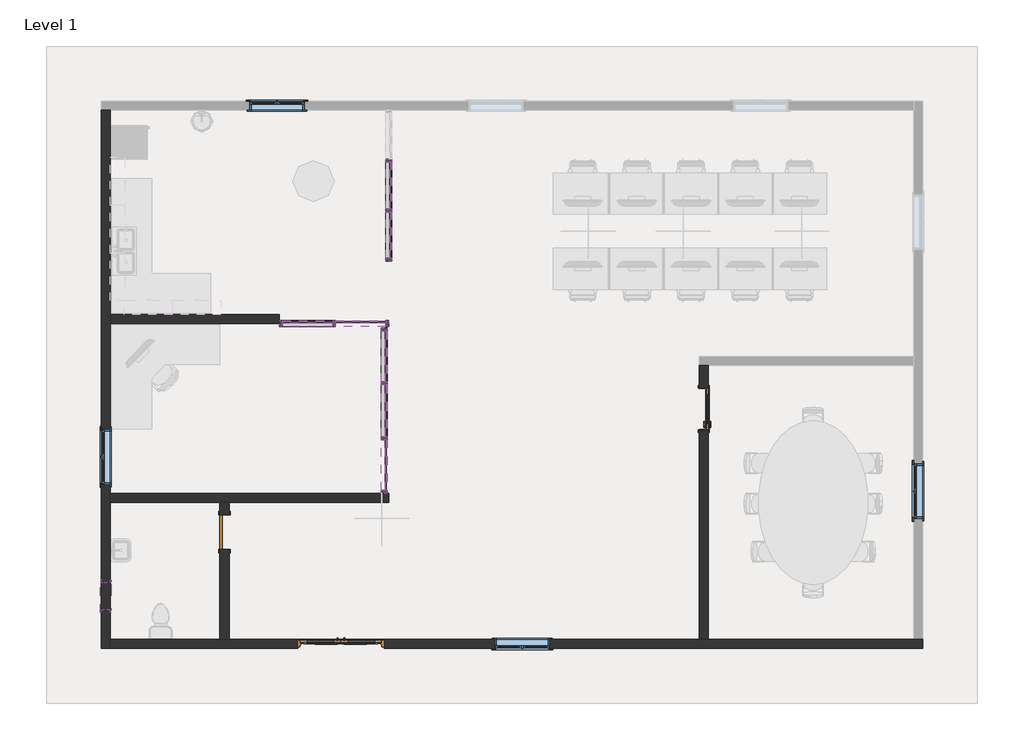
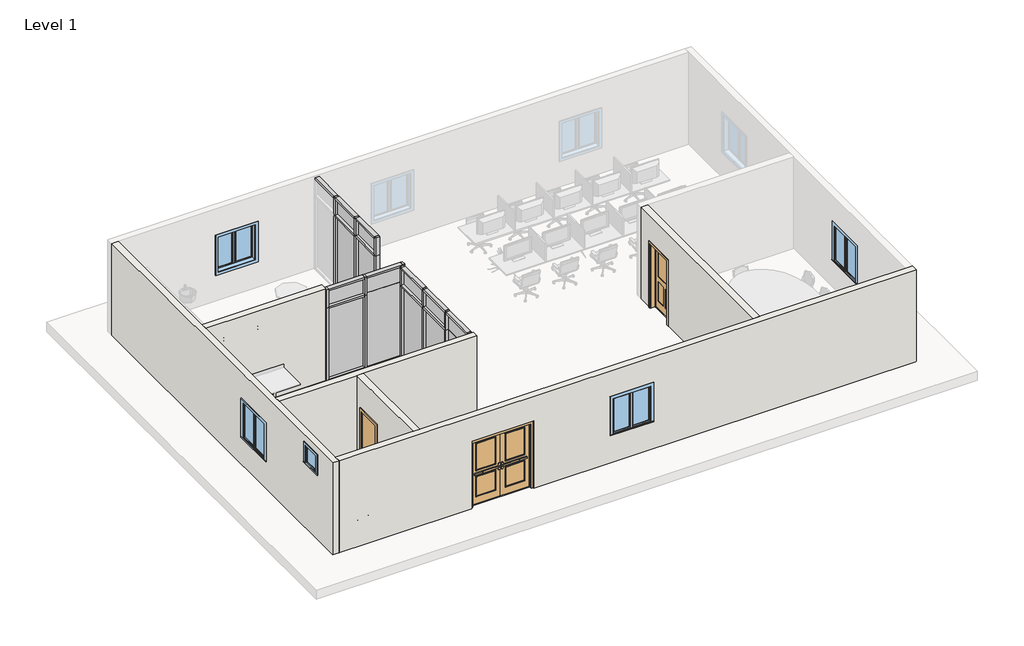
# One storey, part 1 of 2: 38 members, 14 plates, 6 walls, 5 windows, 3 doors.
"""IFC4 building model written with IfcOpenShell, lengths in millimetres."""

from ifc_helpers import new_model, si_unit, frame, origin, origin_with_axes, place, context, project, spatial, polyline, outline, extrude, faceted_brep, transform, mapped, element, save
from components import door_3d09584f, door_6260e01d, door_549a8064, door_95a5efb1, door_1a782ffc, member_f0fea5a5, member_6e77e263, member_47bfaf8a, member_ee409385, member_43f490c4, member_f0038585, member_e3a8255e, member_ffab42ea, member_e6b9f524, member_866a01fa, member_a1c24a98, member_7fa39cca, member_38455fd9, member_afdd3af2, system_panel_glazed_bba99bb7, system_panel_glazed_3d427df9, system_panel_glazed_c20df1b6, system_panel_glazed_49ccfb91, system_panel_glazed_2148303e, system_panel_glazed_80d043f3, system_panel_glazed_79634188, system_panel_glazed_0c115810, system_panel_glazed_47378ea7, system_panel_glazed_21725642, system_panel_glazed_958d1135, system_panel_glazed_0266aec6, system_panel_glazed_6663e6a9, system_panel_glazed_40ca61d7, window_0862ab64, window_e41d21a6

model = new_model("IFC4")

# Units and contexts
model_context = context("Model", 3, world=origin())
ifc_project = project(units=[si_unit("LENGTHUNIT", "METRE", prefix="MILLI")], contexts=[model_context])

# Site, building, storey
site = spatial("IfcSite", under=ifc_project)
building = spatial("IfcBuilding", under=site)
storey = spatial("IfcBuildingStorey", under=building, Name="Level 1", Elevation=0.0)

# Doors
placement = place(None, origin())
door_shape = door_3d09584f(model_context)
element("IfcDoor", 1, ObjectType="36\" x 84\"", at=placement, inside=storey, context=model_context, shape_type="MappedRepresentation", body=[
    mapped(door_shape, transform((-3033.298902, -683.2685778, 0.0), x_axis=(0.0, -1.0, 0.0), y_axis=(1.0, 0.0, 0.0), z_axis=(0.0, 0.0, 1.0))),
])
door_2_shape = door_6260e01d(model_context)
door_3_shape = door_549a8064(model_context)
door_4_shape = door_95a5efb1(model_context)
element("IfcDoor", 2, ObjectType="Door-Exterior-Double-Two_Lite : 72\" x 84\"", at=placement, inside=storey, context=model_context, shape_type="MappedRepresentation", body=[
    mapped(door_2_shape, transform((-11113.673902, -5922.0185778, 0.0), x_axis=(1.0, 0.0, 0.0), y_axis=(0.0, 1.0, 0.0), z_axis=(0.0, 0.0, 1.0))),
    mapped(door_3_shape, transform((-11113.673902, -5922.0185778, 0.0), x_axis=(1.0, 0.0, 0.0), y_axis=(0.0, 1.0, 0.0), z_axis=(0.0, 0.0, 1.0))),
    mapped(door_4_shape, transform((-11113.673902, -5922.0185778, 0.0), x_axis=(1.0, 0.0, 0.0), y_axis=(0.0, 1.0, 0.0), z_axis=(0.0, 0.0, 1.0))),
])
door_5_shape = door_1a782ffc(model_context)
element("IfcDoor", 3, ObjectType="Door-Single-Panel : 30\" x 80\"", at=placement, inside=storey, context=model_context, shape_type="MappedRepresentation", body=[
    mapped(door_5_shape, transform((-13704.473902, -3426.4685778, 0.0), x_axis=(0.0, 1.0, 0.0), y_axis=(-1.0, 0.0, 0.0), z_axis=(0.0, 0.0, 1.0))),
])

# Members
member_shape = member_f0fea5a5(model_context)
element("IfcMember", 4, ObjectType="Rectangular Mullion : 2.5\" x 5\" rectangular", at=placement, inside=storey, context=model_context, shape_type="MappedRepresentation", body=[
    mapped(member_shape, transform((-10148.473902, -107.5352444, 0.0), x_axis=(0.0, -1.0, 0.0), y_axis=(-1.0, 0.0, 0.0), z_axis=(0.0, 0.0, -1.0))),
])
element("IfcMember", 5, ObjectType="Rectangular Mullion : 2.5\" x 5\" rectangular", at=placement, inside=storey, context=model_context, shape_type="MappedRepresentation", body=[
    mapped(member_shape, transform((-10148.473902, -1335.2019111, 0.0), x_axis=(0.0, -1.0, 0.0), y_axis=(-1.0, 0.0, 0.0), z_axis=(0.0, 0.0, -1.0))),
])
element("IfcMember", 6, ObjectType="Rectangular Mullion : 2.5\" x 5\" rectangular", at=placement, inside=storey, context=model_context, shape_type="MappedRepresentation", body=[
    mapped(member_shape, transform((-11266.073902, 1221.7314222, 0.0), x_axis=(1.0, 0.0, 0.0), y_axis=(0.0, -1.0, 0.0), z_axis=(0.0, 0.0, -1.0))),
])
element("IfcMember", 7, ObjectType="Rectangular Mullion : 2.5\" x 5\" rectangular", at=placement, inside=storey, context=model_context, shape_type="MappedRepresentation", body=[
    mapped(member_shape, transform((-10046.873902, 4853.9314222, 0.0), x_axis=(0.0, -1.0, 0.0), y_axis=(-1.0, 0.0, 0.0), z_axis=(0.0, 0.0, -1.0))),
])
element("IfcMember", 8, ObjectType="Rectangular Mullion : 2.5\" x 5\" rectangular", at=placement, inside=storey, context=model_context, shape_type="MappedRepresentation", body=[
    mapped(member_shape, transform((-10046.873902, 3736.3314222, 0.0), x_axis=(0.0, -1.0, 0.0), y_axis=(-1.0, 0.0, 0.0), z_axis=(0.0, 0.0, -1.0))),
])
member_2_shape = member_6e77e263(model_context)
element("IfcMember", 9, ObjectType="Rectangular Mullion : 2.5\" x 5\" rectangular", at=placement, inside=storey, context=model_context, shape_type="MappedRepresentation", body=[
    mapped(member_2_shape, transform((-10148.473902, -107.5352444, 2438.4), x_axis=(0.0, -1.0, 0.0), y_axis=(-1.0, 0.0, 0.0), z_axis=(0.0, 0.0, -1.0))),
])
element("IfcMember", 10, ObjectType="Rectangular Mullion : 2.5\" x 5\" rectangular", at=placement, inside=storey, context=model_context, shape_type="MappedRepresentation", body=[
    mapped(member_2_shape, transform((-10148.473902, -1335.2019111, 2438.4), x_axis=(0.0, -1.0, 0.0), y_axis=(-1.0, 0.0, 0.0), z_axis=(0.0, 0.0, -1.0))),
])
element("IfcMember", 11, ObjectType="Rectangular Mullion : 2.5\" x 5\" rectangular", at=placement, inside=storey, context=model_context, shape_type="MappedRepresentation", body=[
    mapped(member_2_shape, transform((-11266.073902, 1221.7314222, 2438.4), x_axis=(1.0, 0.0, 0.0), y_axis=(0.0, -1.0, 0.0), z_axis=(0.0, 0.0, -1.0))),
])
element("IfcMember", 12, ObjectType="Rectangular Mullion : 2.5\" x 5\" rectangular", at=placement, inside=storey, context=model_context, shape_type="MappedRepresentation", body=[
    mapped(member_2_shape, transform((-10046.873902, 4853.9314222, 2438.4), x_axis=(0.0, -1.0, 0.0), y_axis=(-1.0, 0.0, 0.0), z_axis=(0.0, 0.0, -1.0))),
])
element("IfcMember", 13, ObjectType="Rectangular Mullion : 2.5\" x 5\" rectangular", at=placement, inside=storey, context=model_context, shape_type="MappedRepresentation", body=[
    mapped(member_2_shape, transform((-10046.873902, 3736.3314222, 2438.4), x_axis=(0.0, -1.0, 0.0), y_axis=(-1.0, 0.0, 0.0), z_axis=(0.0, 0.0, -1.0))),
])
member_3_shape = member_47bfaf8a(model_context)
element("IfcMember", 14, ObjectType="Rectangular Mullion : 2.5\" x 5\" rectangular", at=placement, inside=storey, context=model_context, shape_type="MappedRepresentation", body=[
    mapped(member_3_shape, transform((-10148.473902, 1120.1314222, 3048.0), x_axis=(0.0, 1.0, 0.0), y_axis=(-1.0, 0.0, 0.0), z_axis=(0.0, 0.0, 1.0))),
])
element("IfcMember", 15, ObjectType="Rectangular Mullion : 2.5\" x 5\" rectangular", at=placement, inside=storey, context=model_context, shape_type="MappedRepresentation", body=[
    mapped(member_3_shape, transform((-12485.273902, 1221.7314222, 3048.0), x_axis=(-1.0, 0.0, 0.0), y_axis=(0.0, -1.0, 0.0), z_axis=(0.0, 0.0, 1.0))),
])
member_4_shape = member_ee409385(model_context)
element("IfcMember", 16, ObjectType="Rectangular Mullion : 2.5\" x 5\" rectangular", at=placement, inside=storey, context=model_context, shape_type="MappedRepresentation", body=[
    mapped(member_4_shape, transform((-10148.473902, 1120.1314222, 2438.4), x_axis=(0.0, 1.0, 0.0), y_axis=(-1.0, 0.0, 0.0), z_axis=(0.0, 0.0, 1.0))),
])
element("IfcMember", 17, ObjectType="Rectangular Mullion : 2.5\" x 5\" rectangular", at=placement, inside=storey, context=model_context, shape_type="MappedRepresentation", body=[
    mapped(member_4_shape, transform((-12485.273902, 1221.7314222, 2438.4), x_axis=(-1.0, 0.0, 0.0), y_axis=(0.0, -1.0, 0.0), z_axis=(0.0, 0.0, 1.0))),
])
member_5_shape = member_43f490c4(model_context)
element("IfcMember", 18, ObjectType="Rectangular Mullion : 2.5\" x 5\" rectangular", at=placement, inside=storey, context=model_context, shape_type="MappedRepresentation", body=[
    mapped(member_5_shape, transform((-10148.473902, -2499.3685778, 3048.0), x_axis=(0.0, 0.0, 1.0), y_axis=(-1.0, 0.0, 0.0), z_axis=(0.0, -1.0, 0.0))),
])
element("IfcMember", 19, ObjectType="Rectangular Mullion : 2.5\" x 5\" rectangular", at=placement, inside=storey, context=model_context, shape_type="MappedRepresentation", body=[
    mapped(member_5_shape, transform((-10148.473902, -75.7852444, 3048.0), x_axis=(0.0, 0.0, 1.0), y_axis=(-1.0, 0.0, 0.0), z_axis=(0.0, -1.0, 0.0))),
])
element("IfcMember", 20, ObjectType="Rectangular Mullion : 2.5\" x 5\" rectangular", at=placement, inside=storey, context=model_context, shape_type="MappedRepresentation", body=[
    mapped(member_5_shape, transform((-10148.473902, 1056.6314222, 0.0), x_axis=(0.0, 0.0, -1.0), y_axis=(-1.0, 0.0, 0.0), z_axis=(0.0, 1.0, 0.0))),
])
member_6_shape = member_f0038585(model_context)
element("IfcMember", 21, ObjectType="Rectangular Mullion : 2.5\" x 5\" rectangular", at=placement, inside=storey, context=model_context, shape_type="MappedRepresentation", body=[
    mapped(member_6_shape, transform((-10148.473902, -1303.4519111, 3048.0), x_axis=(0.0, 0.0, 1.0), y_axis=(-1.0, 0.0, 0.0), z_axis=(0.0, -1.0, 0.0))),
])
element("IfcMember", 22, ObjectType="Rectangular Mullion : 2.5\" x 5\" rectangular", at=placement, inside=storey, context=model_context, shape_type="MappedRepresentation", body=[
    mapped(member_6_shape, transform((-10148.473902, -139.2852444, 0.0), x_axis=(0.0, 0.0, -1.0), y_axis=(-1.0, 0.0, 0.0), z_axis=(0.0, 1.0, 0.0))),
])
member_7_shape = member_e3a8255e(model_context)
element("IfcMember", 23, ObjectType="Rectangular Mullion : 2.5\" x 5\" rectangular", at=placement, inside=storey, context=model_context, shape_type="MappedRepresentation", body=[
    mapped(member_7_shape, transform((-10148.473902, -75.7852444, 2438.4), x_axis=(0.0, 0.0, 1.0), y_axis=(-1.0, 0.0, 0.0), z_axis=(0.0, -1.0, 0.0))),
])
member_8_shape = member_ffab42ea(model_context)
element("IfcMember", 24, ObjectType="Rectangular Mullion : 2.5\" x 5\" rectangular", at=placement, inside=storey, context=model_context, shape_type="MappedRepresentation", body=[
    mapped(member_8_shape, transform((-10148.473902, -1303.4519111, 2438.4), x_axis=(0.0, 0.0, 1.0), y_axis=(-1.0, 0.0, 0.0), z_axis=(0.0, -1.0, 0.0))),
])
member_9_shape = member_e6b9f524(model_context)
element("IfcMember", 25, ObjectType="Rectangular Mullion : 2.5\" x 5\" rectangular", at=placement, inside=storey, context=model_context, shape_type="MappedRepresentation", body=[
    mapped(member_9_shape, transform((-10110.373902, 1221.7314222, 3048.0), x_axis=(0.0, 0.0, 1.0), y_axis=(0.0, -1.0, 0.0), z_axis=(1.0, 0.0, 0.0))),
])
element("IfcMember", 26, ObjectType="Rectangular Mullion : 2.5\" x 5\" rectangular", at=placement, inside=storey, context=model_context, shape_type="MappedRepresentation", body=[
    mapped(member_9_shape, transform((-11297.823902, 1221.7314222, 3048.0), x_axis=(0.0, 0.0, 1.0), y_axis=(0.0, -1.0, 0.0), z_axis=(1.0, 0.0, 0.0))),
])
element("IfcMember", 27, ObjectType="Rectangular Mullion : 2.5\" x 5\" rectangular", at=placement, inside=storey, context=model_context, shape_type="MappedRepresentation", body=[
    mapped(member_9_shape, transform((-12421.773902, 1221.7314222, 0.0), x_axis=(0.0, 0.0, -1.0), y_axis=(0.0, -1.0, 0.0), z_axis=(-1.0, 0.0, 0.0))),
])
member_10_shape = member_866a01fa(model_context)
element("IfcMember", 28, ObjectType="Rectangular Mullion : 2.5\" x 5\" rectangular", at=placement, inside=storey, context=model_context, shape_type="MappedRepresentation", body=[
    mapped(member_10_shape, transform((-11297.823902, 1221.7314222, 2438.4), x_axis=(0.0, 0.0, 1.0), y_axis=(0.0, -1.0, 0.0), z_axis=(1.0, 0.0, 0.0))),
])
element("IfcMember", 29, ObjectType="Rectangular Mullion : 2.5\" x 5\" rectangular", at=placement, inside=storey, context=model_context, shape_type="MappedRepresentation", body=[
    mapped(member_3_shape, transform((-10148.473902, -2562.8685778, 2438.4), x_axis=(0.0, -1.0, 0.0), y_axis=(-1.0, 0.0, 0.0), z_axis=(0.0, 0.0, -1.0))),
])
element("IfcMember", 30, ObjectType="Rectangular Mullion : 2.5\" x 5\" rectangular", at=placement, inside=storey, context=model_context, shape_type="MappedRepresentation", body=[
    mapped(member_3_shape, transform((-10046.873902, 1221.7314222, 2438.4), x_axis=(1.0, 0.0, 0.0), y_axis=(0.0, -1.0, 0.0), z_axis=(0.0, 0.0, -1.0))),
])
element("IfcMember", 31, ObjectType="Rectangular Mullion : 2.5\" x 5\" rectangular", at=placement, inside=storey, context=model_context, shape_type="MappedRepresentation", body=[
    mapped(member_4_shape, transform((-10148.473902, -2562.8685778, 0.0), x_axis=(0.0, -1.0, 0.0), y_axis=(-1.0, 0.0, 0.0), z_axis=(0.0, 0.0, -1.0))),
])
element("IfcMember", 32, ObjectType="Rectangular Mullion : 2.5\" x 5\" rectangular", at=placement, inside=storey, context=model_context, shape_type="MappedRepresentation", body=[
    mapped(member_4_shape, transform((-10046.873902, 1221.7314222, 0.0), x_axis=(1.0, 0.0, 0.0), y_axis=(0.0, -1.0, 0.0), z_axis=(0.0, 0.0, -1.0))),
])
member_11_shape = member_a1c24a98(model_context)
element("IfcMember", 33, ObjectType="Rectangular Mullion : 2.5\" x 5\" rectangular", at=placement, inside=storey, context=model_context, shape_type="MappedRepresentation", body=[
    mapped(member_11_shape, transform((-10046.873902, 2682.2314222, 3048.0), x_axis=(0.0, 0.0, 1.0), y_axis=(-1.0, 0.0, 0.0), z_axis=(0.0, -1.0, 0.0))),
])
element("IfcMember", 34, ObjectType="Rectangular Mullion : 2.5\" x 5\" rectangular", at=placement, inside=storey, context=model_context, shape_type="MappedRepresentation", body=[
    mapped(member_11_shape, transform((-10046.873902, 4885.6814222, 3048.0), x_axis=(0.0, 0.0, 1.0), y_axis=(-1.0, 0.0, 0.0), z_axis=(0.0, -1.0, 0.0))),
])
member_12_shape = member_7fa39cca(model_context)
element("IfcMember", 35, ObjectType="Rectangular Mullion : 2.5\" x 5\" rectangular", at=placement, inside=storey, context=model_context, shape_type="MappedRepresentation", body=[
    mapped(member_12_shape, transform((-10046.873902, 3768.0814222, 3048.0), x_axis=(0.0, 0.0, 1.0), y_axis=(-1.0, 0.0, 0.0), z_axis=(0.0, -1.0, 0.0))),
])
element("IfcMember", 36, ObjectType="Rectangular Mullion : 2.5\" x 5\" rectangular", at=placement, inside=storey, context=model_context, shape_type="MappedRepresentation", body=[
    mapped(member_11_shape, transform((-10046.873902, 3704.5814222, 0.0), x_axis=(0.0, 0.0, -1.0), y_axis=(-1.0, 0.0, 0.0), z_axis=(0.0, 1.0, 0.0))),
])
element("IfcMember", 37, ObjectType="Rectangular Mullion : 2.5\" x 5\" rectangular", at=placement, inside=storey, context=model_context, shape_type="MappedRepresentation", body=[
    mapped(member_12_shape, transform((-10046.873902, 4822.1814222, 0.0), x_axis=(0.0, 0.0, -1.0), y_axis=(-1.0, 0.0, 0.0), z_axis=(0.0, 1.0, 0.0))),
])
member_13_shape = member_38455fd9(model_context)
element("IfcMember", 38, ObjectType="Rectangular Mullion : 2.5\" x 5\" rectangular", at=placement, inside=storey, context=model_context, shape_type="MappedRepresentation", body=[
    mapped(member_13_shape, transform((-10046.873902, 2682.2314222, 2438.4), x_axis=(0.0, 0.0, 1.0), y_axis=(-1.0, 0.0, 0.0), z_axis=(0.0, -1.0, 0.0))),
])
member_14_shape = member_afdd3af2(model_context)
element("IfcMember", 39, ObjectType="Rectangular Mullion : 2.5\" x 5\" rectangular", at=placement, inside=storey, context=model_context, shape_type="MappedRepresentation", body=[
    mapped(member_14_shape, transform((-10046.873902, 3768.0814222, 2438.4), x_axis=(0.0, 0.0, 1.0), y_axis=(-1.0, 0.0, 0.0), z_axis=(0.0, -1.0, 0.0))),
])
element("IfcMember", 40, ObjectType="Rectangular Mullion : 2.5\" x 5\" rectangular", at=placement, inside=storey, context=model_context, shape_type="MappedRepresentation", body=[
    mapped(member_4_shape, transform((-10046.873902, 2618.7314222, 0.0), x_axis=(0.0, -1.0, 0.0), y_axis=(-1.0, 0.0, 0.0), z_axis=(0.0, 0.0, -1.0))),
])
element("IfcMember", 41, ObjectType="Rectangular Mullion : 2.5\" x 5\" rectangular", at=placement, inside=storey, context=model_context, shape_type="MappedRepresentation", body=[
    mapped(member_3_shape, transform((-10046.873902, 2618.7314222, 2438.4), x_axis=(0.0, -1.0, 0.0), y_axis=(-1.0, 0.0, 0.0), z_axis=(0.0, 0.0, -1.0))),
])

# Plates
system_panel_glazed_shape = system_panel_glazed_bba99bb7(model_context)
element("IfcPlate", 42, ObjectType="System Panel : Glazed", at=placement, inside=storey, context=model_context, shape_type="MappedRepresentation", body=[
    mapped(system_panel_glazed_shape, transform((-10148.473902, 490.4230889, 63.5), x_axis=(0.0, -1.0, 0.0), y_axis=(1.0, 0.0, 0.0), z_axis=(0.0, 0.0, 1.0))),
])
system_panel_glazed_2_shape = system_panel_glazed_3d427df9(model_context)
element("IfcPlate", 43, ObjectType="System Panel : Glazed", at=placement, inside=storey, context=model_context, shape_type="MappedRepresentation", body=[
    mapped(system_panel_glazed_2_shape, transform((-10148.473902, -721.3685778, 63.5), x_axis=(0.0, -1.0, 0.0), y_axis=(1.0, 0.0, 0.0), z_axis=(0.0, 0.0, 1.0))),
])
system_panel_glazed_3_shape = system_panel_glazed_c20df1b6(model_context)
element("IfcPlate", 44, ObjectType="System Panel : Glazed", at=placement, inside=storey, context=model_context, shape_type="MappedRepresentation", body=[
    mapped(system_panel_glazed_3_shape, transform((-10148.473902, 490.4230889, 2470.15), x_axis=(0.0, -1.0, 0.0), y_axis=(1.0, 0.0, 0.0), z_axis=(0.0, 0.0, 1.0))),
])
system_panel_glazed_4_shape = system_panel_glazed_49ccfb91(model_context)
element("IfcPlate", 45, ObjectType="System Panel : Glazed", at=placement, inside=storey, context=model_context, shape_type="MappedRepresentation", body=[
    mapped(system_panel_glazed_4_shape, transform((-10148.473902, -721.3685778, 2470.15), x_axis=(0.0, -1.0, 0.0), y_axis=(1.0, 0.0, 0.0), z_axis=(0.0, 0.0, 1.0))),
])
system_panel_glazed_5_shape = system_panel_glazed_2148303e(model_context)
element("IfcPlate", 46, ObjectType="System Panel : Glazed", at=placement, inside=storey, context=model_context, shape_type="MappedRepresentation", body=[
    mapped(system_panel_glazed_5_shape, transform((-11859.798902, 1221.7314222, 63.5), x_axis=(1.0, 0.0, 0.0), y_axis=(0.0, 1.0, 0.0), z_axis=(0.0, 0.0, 1.0))),
])
system_panel_glazed_6_shape = system_panel_glazed_80d043f3(model_context)
element("IfcPlate", 47, ObjectType="System Panel : Glazed", at=placement, inside=storey, context=model_context, shape_type="MappedRepresentation", body=[
    mapped(system_panel_glazed_6_shape, transform((-11859.798902, 1221.7314222, 2470.15), x_axis=(1.0, 0.0, 0.0), y_axis=(0.0, 1.0, 0.0), z_axis=(0.0, 0.0, 1.0))),
])
system_panel_glazed_7_shape = system_panel_glazed_79634188(model_context)
element("IfcPlate", 48, ObjectType="System Panel : Glazed", at=placement, inside=storey, context=model_context, shape_type="MappedRepresentation", body=[
    mapped(system_panel_glazed_7_shape, transform((-10672.348902, 1221.7314222, 2438.4), x_axis=(1.0, 0.0, 0.0), y_axis=(0.0, 1.0, 0.0), z_axis=(0.0, 0.0, 1.0))),
])
system_panel_glazed_8_shape = system_panel_glazed_0c115810(model_context)
element("IfcPlate", 49, ObjectType="System Panel : Glazed", at=placement, inside=storey, context=model_context, shape_type="MappedRepresentation", body=[
    mapped(system_panel_glazed_8_shape, transform((-10672.348902, 1221.7314222, 0.0), x_axis=(1.0, 0.0, 0.0), y_axis=(0.0, 1.0, 0.0), z_axis=(0.0, 0.0, 1.0))),
])
system_panel_glazed_9_shape = system_panel_glazed_47378ea7(model_context)
element("IfcPlate", 50, ObjectType="System Panel : Glazed", at=placement, inside=storey, context=model_context, shape_type="MappedRepresentation", body=[
    mapped(system_panel_glazed_9_shape, transform((-10148.473902, -1933.1602444, 0.0), x_axis=(0.0, -1.0, 0.0), y_axis=(1.0, 0.0, 0.0), z_axis=(0.0, 0.0, 1.0))),
])
system_panel_glazed_10_shape = system_panel_glazed_21725642(model_context)
element("IfcPlate", 51, ObjectType="System Panel : Glazed", at=placement, inside=storey, context=model_context, shape_type="MappedRepresentation", body=[
    mapped(system_panel_glazed_10_shape, transform((-10148.473902, -1933.1602444, 2438.4), x_axis=(0.0, -1.0, 0.0), y_axis=(1.0, 0.0, 0.0), z_axis=(0.0, 0.0, 1.0))),
])
system_panel_glazed_11_shape = system_panel_glazed_958d1135(model_context)
element("IfcPlate", 52, ObjectType="System Panel : Glazed", at=placement, inside=storey, context=model_context, shape_type="MappedRepresentation", body=[
    mapped(system_panel_glazed_11_shape, transform((-10046.873902, 3193.4064222, 63.5), x_axis=(0.0, -1.0, 0.0), y_axis=(1.0, 0.0, 0.0), z_axis=(0.0, 0.0, 1.0))),
])
system_panel_glazed_12_shape = system_panel_glazed_0266aec6(model_context)
element("IfcPlate", 53, ObjectType="System Panel : Glazed", at=placement, inside=storey, context=model_context, shape_type="MappedRepresentation", body=[
    mapped(system_panel_glazed_12_shape, transform((-10046.873902, 4295.1314222, 63.5), x_axis=(0.0, -1.0, 0.0), y_axis=(1.0, 0.0, 0.0), z_axis=(0.0, 0.0, 1.0))),
])
system_panel_glazed_13_shape = system_panel_glazed_6663e6a9(model_context)
element("IfcPlate", 54, ObjectType="System Panel : Glazed", at=placement, inside=storey, context=model_context, shape_type="MappedRepresentation", body=[
    mapped(system_panel_glazed_13_shape, transform((-10046.873902, 3193.4064222, 2470.15), x_axis=(0.0, -1.0, 0.0), y_axis=(1.0, 0.0, 0.0), z_axis=(0.0, 0.0, 1.0))),
])
system_panel_glazed_14_shape = system_panel_glazed_40ca61d7(model_context)
element("IfcPlate", 55, ObjectType="System Panel : Glazed", at=placement, inside=storey, context=model_context, shape_type="MappedRepresentation", body=[
    mapped(system_panel_glazed_14_shape, transform((-10046.873902, 4295.1314222, 2470.15), x_axis=(0.0, -1.0, 0.0), y_axis=(1.0, 0.0, 0.0), z_axis=(0.0, 0.0, 1.0))),
])

# Walls
element("IfcWall", 56, ObjectType="Generic - 8\"", at=placement, inside=storey, context=model_context, shape_type="Brep", body=[
    faceted_brep([(-16244.473902, -6017.2685778, 0.0), (-16244.473902, -5814.0685778, 0.0), (-16244.473902, -2766.0685778, 0.0), (-16244.473902, -2562.8685778, 0.0), (-16244.473902, 1221.7314222, 0.0), (-16244.473902, 1424.9314222, 0.0), (-16244.473902, 5971.5314222, 0.0), (-16244.473902, 5971.5314222, 3048.0), (-16244.473902, 1424.9314222, 3048.0), (-16244.473902, 1221.7314222, 3048.0), (-16244.473902, -2562.8685778, 3048.0), (-16244.473902, -2766.0685778, 3048.0), (-16244.473902, -5814.0685778, 3048.0), (-16244.473902, -6017.2685778, 3048.0), (-16244.473902, -1140.4685778, 2133.6), (-16244.473902, -1140.4685778, 914.4), (-16244.473902, -2359.6685778, 914.4), (-16244.473902, -2359.6685778, 2133.6), (-16244.473902, -4544.0685778, 2768.6), (-16244.473902, -4544.0685778, 2159.0), (-16244.473902, -5153.6685778, 2159.0), (-16244.473902, -5153.6685778, 2768.6), (-16447.673902, -6017.2685778, 0.0), (-16447.673902, -6017.2685778, 3048.0), (-16447.673902, 5971.5314222, 3048.0), (-16447.673902, 5971.5314222, 0.0), (-16447.673902, -1140.4685778, 2133.6), (-16447.673902, -2359.6685778, 2133.6), (-16447.673902, -2359.6685778, 914.4), (-16447.673902, -1140.4685778, 914.4), (-16447.673902, -4544.0685778, 2768.6), (-16447.673902, -5153.6685778, 2768.6), (-16447.673902, -5153.6685778, 2159.0), (-16447.673902, -4544.0685778, 2159.0)], [[[0, 1, 2, 3, 4, 5, 6, 7, 8, 9, 10, 11, 12, 13], [14, 15, 16, 17], [18, 19, 20, 21]], [[22, 23, 24, 25], [26, 27, 28, 29], [30, 31, 32, 33]], [[6, 5, 4, 3, 2, 1, 0, 22, 25]], [[13, 12, 11, 10, 9, 8, 7, 24, 23]], [[0, 13, 23, 22]], [[7, 6, 25, 24]], [[15, 14, 26, 29]], [[16, 15, 29, 28]], [[17, 16, 28, 27]], [[14, 17, 27, 26]], [[19, 18, 30, 33]], [[20, 19, 33, 32]], [[21, 20, 32, 31]], [[18, 21, 31, 30]]]),
])
element("IfcWall", 57, ObjectType="Generic - 8\"", at=placement, inside=storey, context=model_context, shape_type="Brep", body=[
    faceted_brep([(-16244.473902, -5814.0685778, 3048.0), (-13806.073902, -5814.0685778, 3048.0), (-13602.873902, -5814.0685778, 3048.0), (-3138.073902, -5814.0685778, 3048.0), (-2934.873902, -5814.0685778, 3048.0), (1637.126098, -5814.0685778, 3048.0), (1840.326098, -5814.0685778, 3048.0), (1840.326098, -5814.0685778, 0.0), (1637.126098, -5814.0685778, 0.0), (-2934.873902, -5814.0685778, 0.0), (-3138.073902, -5814.0685778, 0.0), (-10148.473902, -5814.0685778, 0.0), (-10148.473902, -5814.0685778, 2235.2), (-12078.873902, -5814.0685778, 2235.2), (-12078.873902, -5814.0685778, 0.0), (-13602.873902, -5814.0685778, 0.0), (-13806.073902, -5814.0685778, 0.0), (-16244.473902, -5814.0685778, 0.0), (-7684.673902, -5814.0685778, 2133.6), (-7684.673902, -5814.0685778, 914.4), (-6465.473902, -5814.0685778, 914.4), (-6465.473902, -5814.0685778, 2133.6), (1840.326098, -6017.2685778, 3048.0), (-16244.473902, -6017.2685778, 3048.0), (-16244.473902, -6017.2685778, 0.0), (-12078.873902, -6017.2685778, 0.0), (-12078.873902, -6017.2685778, 2235.2), (-10148.473902, -6017.2685778, 2235.2), (-10148.473902, -6017.2685778, 0.0), (1840.326098, -6017.2685778, 0.0), (-7684.673902, -6017.2685778, 2133.6), (-6465.473902, -6017.2685778, 2133.6), (-6465.473902, -6017.2685778, 914.4), (-7684.673902, -6017.2685778, 914.4)], [[[0, 1, 2, 3, 4, 5, 6, 7, 8, 9, 10, 11, 12, 13, 14, 15, 16, 17], [18, 19, 20, 21]], [[22, 23, 24, 25, 26, 27, 28, 29], [30, 31, 32, 33]], [[7, 29, 28, 11, 10, 9, 8]], [[24, 17, 16, 15, 14, 25]], [[6, 5, 4, 3, 2, 1, 0, 23, 22]], [[7, 6, 22, 29]], [[0, 17, 24, 23]], [[27, 12, 11, 28]], [[12, 27, 26, 13]], [[13, 26, 25, 14]], [[19, 18, 30, 33]], [[20, 19, 33, 32]], [[21, 20, 32, 31]], [[18, 21, 31, 30]]]),
])
element("IfcWall", 58, ObjectType="Generic - 8\"", at=placement, inside=storey, context=model_context, shape_type="SweptSolid", body=[
    extrude(outline(polyline([(-5814.0685778, 3048.0), (281.9314222, 3048.0), (281.9314222, 0.0), (-200.6685778, 0.0), (-200.6685778, 2159.0), (-1165.8685778, 2159.0), (-1165.8685778, 0.0), (-5814.0685778, 0.0), (-5814.0685778, 3048.0)])), frame((-3138.073902, 0.0, 0.0), z_axis=(1.0, 0.0, 0.0), x_axis=(0.0, 1.0, 0.0)), (0.0, 0.0, 1.0), 203.2),
])
element("IfcWall", 59, ObjectType="Generic - 8\"", at=placement, inside=storey, context=model_context, shape_type="SweptSolid", body=[
    extrude(outline(polyline([(-2766.0685778, 0.0), (-3045.4685778, 0.0), (-3045.4685778, 2032.0), (-3807.4685778, 2032.0), (-3807.4685778, 0.0), (-5814.0685778, 0.0), (-5814.0685778, 3048.0), (-2766.0685778, 3048.0), (-2766.0685778, 0.0)])), frame((-13806.073902, 0.0, 0.0), z_axis=(1.0, 0.0, 0.0), x_axis=(0.0, 1.0, 0.0)), (0.0, 0.0, 1.0), 203.2),
])
element("IfcWall", 60, ObjectType="Generic - 8\"", at=placement, inside=storey, context=model_context, shape_type="Brep", body=[
    faceted_brep([(-10046.873902, -2562.8685778, 0.0), (-16244.473902, -2562.8685778, 0.0), (-16244.473902, -2562.8685778, 3048.0), (-10046.873902, -2562.8685778, 3048.0), (-10046.873902, -2766.0685778, 0.0), (-10046.873902, -2766.0685778, 3048.0), (-13602.873902, -2766.0685778, 3048.0), (-13806.073902, -2766.0685778, 3048.0), (-16244.473902, -2766.0685778, 3048.0), (-16244.473902, -2766.0685778, 0.0), (-13806.073902, -2766.0685778, 0.0), (-13602.873902, -2766.0685778, 0.0)], [[[0, 1, 2, 3]], [[4, 5, 6, 7, 8, 9, 10, 11]], [[1, 0, 4, 11, 10, 9]], [[3, 2, 8, 7, 6, 5]], [[0, 3, 5, 4]], [[2, 1, 9, 8]]]),
])
element("IfcWall", 61, ObjectType="Generic - 8\"", at=placement, inside=storey, context=model_context, shape_type="SweptSolid", body=[
    extrude(outline(polyline([(-12485.273902, 1221.7314222), (-16244.473902, 1221.7314222), (-16244.473902, 1424.9314222), (-12485.273902, 1424.9314222), (-12485.273902, 1221.7314222)])), origin_with_axes(), (0.0, 0.0, 1.0), 3048.0),
])

# Windows
window_shape = window_0862ab64(model_context)
element("IfcWindow", 62, ObjectType="Casement Dbl with Trim : 48\" x 48\"", at=placement, inside=storey, context=model_context, shape_type="MappedRepresentation", body=[
    mapped(window_shape, transform((-12536.073902, 6054.0814222, 0.0), x_axis=(1.0, 0.0, 0.0), y_axis=(0.0, 1.0, 0.0), z_axis=(0.0, 0.0, 1.0))),
])
element("IfcWindow", 63, ObjectType="Casement Dbl with Trim : 48\" x 48\"", at=placement, inside=storey, context=model_context, shape_type="MappedRepresentation", body=[
    mapped(window_shape, transform((1757.776098, -2512.0685778, 0.0), x_axis=(0.0, 1.0, 0.0), y_axis=(-1.0, 0.0, 0.0), z_axis=(0.0, 0.0, 1.0))),
])
element("IfcWindow", 64, ObjectType="Casement Dbl with Trim : 48\" x 48\"", at=placement, inside=storey, context=model_context, shape_type="MappedRepresentation", body=[
    mapped(window_shape, transform((-7075.073902, -5896.6185778, 0.0), x_axis=(-1.0, 0.0, 0.0), y_axis=(0.0, -1.0, 0.0), z_axis=(0.0, 0.0, 1.0))),
])
element("IfcWindow", 65, ObjectType="Casement Dbl with Trim : 48\" x 48\"", at=placement, inside=storey, context=model_context, shape_type="MappedRepresentation", body=[
    mapped(window_shape, transform((-16327.023902, -1750.0685778, 0.0), x_axis=(0.0, 1.0, 0.0), y_axis=(-1.0, 0.0, 0.0), z_axis=(0.0, 0.0, 1.0))),
])
window_2_shape = window_e41d21a6(model_context)
element("IfcWindow", 66, ObjectType="Transom with Trim : 24\" x 24\"", at=placement, inside=storey, context=model_context, shape_type="MappedRepresentation", body=[
    mapped(window_2_shape, transform((-16346.073902, -4810.7685778, 0.0), x_axis=(0.0, 1.0, 0.0), y_axis=(-1.0, 0.0, 0.0), z_axis=(0.0, 0.0, 1.0))),
])

save(model, "model.ifc")

# Revit data of these elements
# Type "36\" x 84\""
#   Type Mark = "11"
#   Assembly Code = "B2030100"
#   Analytic Construction = "French door, wood frame with single glass"
#   Top Rail = 0' - 4 3/4"
#   Threshold Offset [instance default] = 0' - 0 1/2"
#   Thickness = 0' - 1 3/8"
#   Thermal Resistance (R) = 1.0696 (h·ft²·°F)/BTU
#   Swing Angle [instance default] = 90.00°
#   Stiles = 0' - 4 3/4"
#   Rough Width = 3' - 2"
#   Rough Height = 7' - 1"
#   Lock Rail = 0' - 7 1/8"
#   Height = 7' - 0"
#   Width = 3' - 0"
#   Heat Transfer Coefficient (U) = 0.9350 BTU/(h·ft²·°F)
#   Door Offset [instance default] = 0' - 0"
#   Bottom Rail = 0' - 9 1/2"
#   Threshold [instance default] = yes
#   Function = 1
#   Exterior Trim [instance default] = yes
#   Trim Material = Cherry
#   Threshold Material = Cherry
#   Panel Material = Cherry
#   Glazing = Glass
#   Frame Material = Cherry
#   Door Handle Material = Aluminum
#   Visual Light Transmittance = 0
#   Solar Heat Gain Coefficient = 0
#   Wall Closure = (empty or 0)
#   Construction Type = (empty or 0)
# Type "Door-Exterior-Double-Two_Lite : 72\" x 84\""
#   Type Mark = "8"
#   Assembly Code = "B2030100"
#   Analytic Construction = "Metal frame, double glass door"
#   Top Rail = 0' - 4 5/8"
#   Threshold Length [instance default] = 6' - 4"
#   Threshold Offset [instance default] = 0' - 0 1/2"
#   Thickness = 0' - 1 3/4"
#   Thermal Resistance (R) = 1.3794 (h·ft²·°F)/BTU
#   Swing Angle [instance default] = 90.00°
#   Strike Height = 3' - 4"
#   Stiles = 0' - 6"
#   SinglePanelWidth = 3' - 0"
#   Rough Width [instance default] = 6' - 4"
#   Rough Height [instance default] = 7' - 4"
#   MFOpeningHeight [instance default] = 0' - 4"
#   MFOpeningWidth [instance default] = 0' - 4"
#   Lock Rail = 0' - 8"
#   Inset Calculate [instance default] = 0' - 4"
#   Masonry Inset [instance default] = 0' - 1"
#   Height = 7' - 0"
#   Width = 6' - 0"
#   Heat Transfer Coefficient (U) = 0.7250 BTU/(h·ft²·°F)
#   Glass Thickness = 0' - 0 3/4"
#   Masonry Frame Depth = 0' - 5 3/4"
#   Bottom Rail = 0' - 10"
#   Threshold [instance default] = yes
#   Masonry Frame [instance default] = yes
#   Function = 1
#   Dry Wall Frame [instance default] = no
#   Threshold Material = none
#   Panic Bar Material = Metal - Stainless Steel
#   Panel Material = Metal - Painted - Grey
#   Glass Stop Material = Metal - Painted - Grey
#   Frame Material = Metal - Painted - Grey
#   Exterior Pull Material = Metal - Stainless Steel
#   Visual Light Transmittance = 0
#   Solar Heat Gain Coefficient = 0
#   Wall Closure = (empty or 0)
# Type "Door-Single-Panel : 30\" x 80\""
#   Type Mark = "10"
#   Construction Type Id = "DOOR"
#   Assembly Code = "C1020300"
#   Analytic Construction = "Wooden"
#   Thickness = 0' - 2"
#   Thermal Resistance (R) = 2.5876 (h·ft²·°F)/BTU
#   Swing Angle [instance default] = 90.00°
#   Heat Transfer Coefficient (U) = 0.3865 BTU/(h·ft²·°F)
#   Height = 6' - 8"
#   Trim Projection Ext = 0' - 1"
#   Trim Projection Int = 0' - 1"
#   Trim Width = 0' - 3"
#   Width = 2' - 6"
#   Define Thermal Properties by = 1
#   Panel Material = Wood - Birch - Solid Stained Light Low Gloss
#   Trim Material = Paint - Sienna
#   Visual Light Transmittance = 0
#   Solar Heat Gain Coefficient = 0
#   Function = (empty or 0)
#   Wall Closure = (empty or 0)
# Type "Rectangular Mullion : 2.5\" x 5\" rectangular"
#   built-in parameter 1007304 = 0.416667 (stored number, unit not read)
#   built-in parameter 1007301 = 0.104167 (stored number, unit not read)
#   built-in parameter 1007300 = 0.104167 (stored number, unit not read)
# Type "System Panel : Glazed"
#   Construction Type Id = "GSP4R"
#   Analytic Construction = "1/8 in Pilkington single glazing"
#   Visual Light Transmittance = 0.9
#   Solar Heat Gain Coefficient = 0.86
#   Heat Transfer Coefficient (U) = 1.18115 BTU/(h·ft²·°F)
# Type "Generic - 8\""
#   Assembly Code = "B2010"
#   Layers, outside or top first: 0' - 8" "WALL 1" (function 1)
# Type "Casement Dbl with Trim : 48\" x 48\""
#   Type Mark = "10"
#   Construction Type Id = "GSP4R"
#   Assembly Code = "B2020100"
#   Analytic Construction = "1/8 in Pilkington single glazing"
#   Visual Light Transmittance = 0.9
#   Solar Heat Gain Coefficient = 0.78
#   Heat Transfer Coefficient (U) = 0.6496 BTU/(h·ft²·°F)
#   Height = 4' - 0"
#   Default Sill Height = 3' - 0"
#   Trim Projection - Ext. = 0' - 0 1/2"
#   Trim Projection - Int. = 0' - 0 3/4"
#   Trim Width - Exterior = 0' - 3 1/2"
#   Trim Width - Interior = 0' - 3 1/2"
#   Width = 4' - 0"
#   Window Inset = 0' - 0 3/4"
#   Define Thermal Properties by = 1
#   Glass Pane Material = Glass
#   Sash Material = Sash
#   Trim Exterior Material = Trim
#   Trim Interior Material = Trim
#   Wall Closure = (empty or 0)
# Type "Transom with Trim : 24\" x 24\""
#   Type Mark = "13"
#   Construction Type Id = "GSP4R"
#   Assembly Code = "B2020100"
#   Analytic Construction = "1/8 in Pilkington single glazing"
#   Visual Light Transmittance = 0.9
#   Solar Heat Gain Coefficient = 0.78
#   Heat Transfer Coefficient (U) = 0.6496 BTU/(h·ft²·°F)
#   Height = 2' - 0"
#   Default Sill Height = 7' - 1"
#   Trim Projection - Ext. = 0' - 0 1/2"
#   Trim Projection - Int. = 0' - 0 3/4"
#   Trim Width - Exterior = 0' - 3 1/2"
#   Trim Width - Interior = 0' - 3 1/2"
#   Width = 2' - 0"
#   Window Inset = 0' - 0 3/4"
#   Define Thermal Properties by = 1
#   Glass Pane Material = Glass
#   Sash Material = Sash
#   Trim Exterior Material = Trim
#   Trim Interior Material = Trim
#   Wall Closure = (empty or 0)
# Element 1 (IfcDoor, "36\" x 84\"")
#   Threshold Offset = 0' - 0 1/2"
#   Swing Angle = 90.00°
#   Door Offset = 0' - 0"
#   Threshold = yes
#   Exterior Trim = yes
#   Phase Created = New Construction
#   Materials on its faces: "Cherry", "Aluminum", "Glass"
# Element 2 (IfcDoor, "Door-Exterior-Double-Two_Lite : 72\" x 84\"")
#   Threshold Offset = 0' - 0 1/2"
#   Threshold Length = 6' - 4"
#   Swing Angle = 90.00°
#   Rough Width = 6' - 4"
#   Rough Height = 7' - 4"
#   Masonry Inset = 0' - 1"
#   MFOpeningWidth = 0' - 4"
#   MFOpeningHeight = 0' - 4"
#   Inset Calculate = 0' - 4"
#   Threshold = yes
#   Masonry Frame = yes
#   Dry Wall Frame = no
#   Phase Created = New Construction
#   Materials on its faces: "Metal - Painted - Grey", "Metal - Stainless Steel", "Glass"
# Element 3 (IfcDoor, "Door-Single-Panel : 30\" x 80\"")
#   Swing Angle = 90.00°
#   Phase Created = New Construction
#   Materials on its faces: "Paint - Sienna", "Wood - Birch - Solid Stained Light Low Gloss"
# Elements 4, 5, 6, 7, 8, 9, 10, 11, 12, 13, 14, 15, 16, 17, 18, 19, 20, 21, 22, 23, 24, 25, 26, 27, 28, 29, 30, 31, 32, 33, 34, 35, 36, 37, 38, 39, 40, 41 (IfcMember, "Rectangular Mullion : 2.5\" x 5\" rectangular")
#   Phase Created = New Construction
#   Materials on its faces: "Aluminum"
# Elements 42, 43, 44, 45, 46, 47, 48, 49, 50, 51, 52, 53, 54, 55 (IfcPlate, "System Panel : Glazed")
#   Phase Created = New Construction
#   Materials on its faces: "Glass"
# Elements 56, 57, 58, 59, 60, 61 (IfcWall, "Generic - 8\"")
#   Top Offset = 0' - 0"
#   Base Offset = 0' - 0"
#   Unconnected Height = 10' - 0"
#   wall height = 10' - 0"
#   Phase Created = New Construction
#   Base Constraint = Level 1
#   Materials on its faces: "WALL 1"
# Element 62 (IfcWindow, "Casement Dbl with Trim : 48\" x 48\"")
#   Mark = "1"
#   Phase Created = New Construction
#   Materials on its faces: "Sash", "Trim", "Glass"
# Element 63 (IfcWindow, "Casement Dbl with Trim : 48\" x 48\"")
#   Mark = "5"
#   Phase Created = New Construction
#   Materials on its faces: "Sash", "Trim", "Glass"
# Element 64 (IfcWindow, "Casement Dbl with Trim : 48\" x 48\"")
#   Mark = "6"
#   Phase Created = New Construction
#   Materials on its faces: "Sash", "Trim", "Glass"
# Element 65 (IfcWindow, "Casement Dbl with Trim : 48\" x 48\"")
#   Mark = "7"
#   Phase Created = New Construction
#   Materials on its faces: "Sash", "Trim", "Glass"
# Element 66 (IfcWindow, "Transom with Trim : 24\" x 24\"")
#   Mark = "8"
#   Phase Created = New Construction
#   Materials on its faces: "Sash", "Trim", "Glass"
# Materials
#   "Cherry": class "Wood", colour RGB 226 177 128, transparency 0, Description = "Prunus Serotina", Cost = 0
#   "Glass": class "Glass", colour RGB 0 128 192, transparency 0.75, Description = "Soda Lime Glass", Cost = 0
#   "Aluminum": class "Metal", colour RGB 247 247 247, transparency 0, Description = "Aluminum 6061", Cost = 0
#   "Metal - Stainless Steel": class "Metal", colour RGB 247 247 247, transparency 0
#   "Metal - Painted - Grey": class "Paint", colour RGB 104 104 104, transparency 0, Cost = 0
#   "Wood - Birch - Solid Stained Light Low Gloss": class "Wood", colour RGB 210 159 95, transparency 0, Cost = 0
#   "Paint - Sienna": colour RGB 118 70 51, transparency 0, Cost = 0
#   "WALL 1": class "Generic", colour RGB 120 120 120, transparency 0, Cost = 0
#   "Sash": class "Wood", colour RGB 224 178 126, transparency 0
#   "Trim": class "Wood", colour RGB 224 178 126, transparency 0
